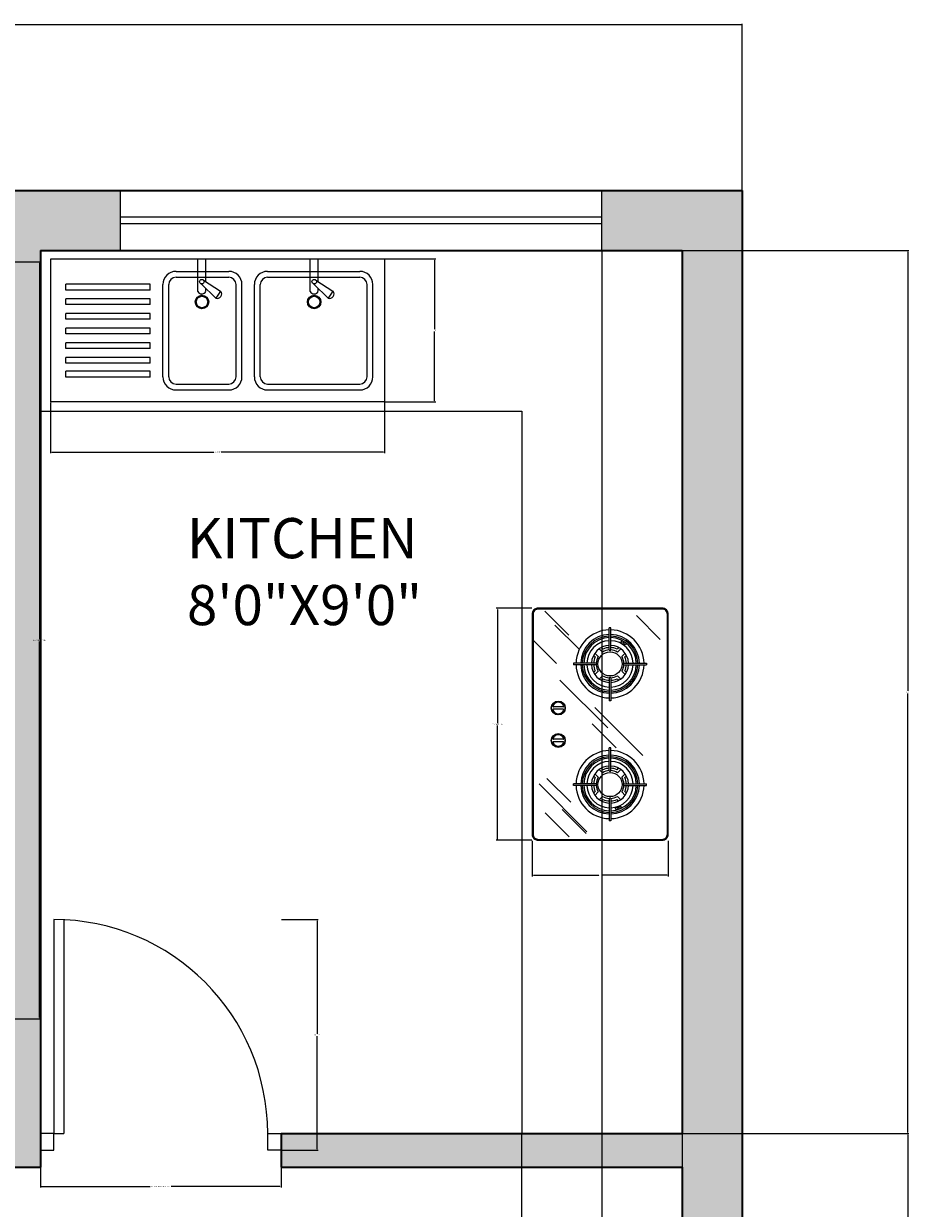
# Model space of a CAD drawing. Units: inches. Extents: x 126 to 477, y -70 to 465.
# Tile 5 of 5: x 344 to 477, y 288 to 465. Entities that reach past the tile are written whole.
import ezdxf

# ---------------------------------------------------------------- set-up
doc = ezdxf.new("R2010")
doc.units = ezdxf.units.IN
for name, color, linetype, lineweight in [('A-ANNO-DIMS', 2, 'Continuous', 18), ('A-AREA-IDEN', 7, 'Continuous', 20), ('A-DOOR', 4, 'Continuous', 20), ('A-EQPM', 9, 'Continuous', 18), ('A-FLOR-CASE', 8, 'Continuous', 25), ('A-FLOR-FIXT', 8, 'Continuous', 18), ('A-GLAZ', 4, 'Continuous', 18), ('A-WALL', 7, 'Continuous', 35), ('A-WALL-PATT', 252, 'Continuous', 13)]:
    doc.layers.add(name, color=color, linetype=linetype, lineweight=lineweight)
doc.styles.get("Standard").update_dxf_attribs({"font": 'arial.ttf'})
doc.dimstyles.get("Standard").update_dxf_attribs({"dimtxt": 0.18, "dimasz": 0.18, "dimexe": 0.18, "dimexo": 0.0625, "dimgap": 0.09, "dimtad": 0, "dimtih": 1, "dimtoh": 1, "dimdec": 4, "dimzin": 0, "dimdsep": 46, "dimtxsty": 'Standard', "dimcen": 0.09, "dimadec": 0, "dimazin": 0, "dimtfac": 1, "dimtdec": 4, "dimtofl": 0, "dimtmove": 0, "dimatfit": 3, "dimfxl": 1, "dimtolj": 1, "dimtzin": 0, "dimarcsym": 0})

# ---------------------------------------------------------------- blocks, each defined once
blk = doc.blocks.new('A$C6CB038CA')
for p, q in [((0, 0), (0, 488.5)), ((0, 488.5), (1140.7, 488.5)), ((502.8, 377.5), (502.8, 488.5)), ((529.8, 412.8), (529.8, 488.5)), ((886.8, 377.5), (886.8, 488.5)), ((913.8, 412.8), (913.8, 488.5)), ((1140.7, 488.5), (1140.7, 0)), ((428.4, 445.8), (608.4, 445.8)), ((740.8, 445.8), (1055.8, 445.8)), ((428.4, 425.8), (608.4, 425.8)), ((521.9, 415.4), (580.3, 378.4)), ((740.8, 425.8), (1055.8, 425.8)), ((906, 415.4), (964.3, 378.4)), ((52.2, 382.1), (52.2, 402.1)), ((339.4, 402.1), (52.2, 402.1)), ((339.4, 382.1), (52.2, 382.1)), ((339.4, 382.1), (339.4, 402.1)), ((383.4, 85.8), (383.4, 400.8)), ((403.4, 85.8), (403.4, 400.8)), ((563.7, 353.9), (514.9, 402.4)), ((529.8, 377.6), (529.8, 387.6)), ((580.3, 378.4), (563.7, 353.9)), ((633.4, 85.8), (633.4, 400.8)), ((653.4, 85.8), (653.4, 400.8)), ((695.8, 85.8), (695.8, 400.8)), ((715.8, 85.8), (715.8, 400.8)), ((947.8, 353.9), (899, 402.4)), ((913.8, 377.6), (913.8, 387.6)), ((964.3, 378.4), (947.8, 353.9)), ((1080.8, 85.8), (1080.8, 400.8)), ((1100.8, 85.8), (1100.8, 400.8)), ((52.2, 332.1), (52.2, 352.1)), ((339.4, 352.1), (52.2, 352.1)), ((339.4, 332.1), (52.2, 332.1)), ((339.4, 332.1), (339.4, 352.1)), ((52.2, 282.1), (52.2, 302.1)), ((339.4, 302.1), (52.2, 302.1)), ((339.4, 282.1), (339.4, 302.1)), ((339.4, 282.1), (52.2, 282.1)), ((52.2, 232.1), (52.2, 252.1)), ((339.4, 252.1), (52.2, 252.1)), ((339.4, 232.1), (339.4, 252.1)), ((339.4, 232.1), (52.2, 232.1)), ((52.2, 182.1), (52.2, 202.1)), ((339.4, 202.1), (52.2, 202.1)), ((339.4, 182.1), (52.2, 182.1)), ((339.4, 182.1), (339.4, 202.1)), ((52.2, 132.1), (52.2, 152.1)), ((339.4, 152.1), (52.2, 152.1)), ((339.4, 132.1), (52.2, 132.1)), ((339.4, 132.1), (339.4, 152.1)), ((52.2, 84.8), (52.2, 104.8)), ((339.4, 104.8), (52.2, 104.8)), ((339.4, 84.8), (52.2, 84.8)), ((339.4, 84.8), (339.4, 104.8)), ((428.4, 60.8), (608.4, 60.8)), ((428.4, 40.8), (608.4, 40.8)), ((740.8, 60.8), (1055.8, 60.8)), ((740.8, 40.8), (1055.8, 40.8)), ((1140.7, 0), (0, 0))]:
    blk.add_line(p, q)
for centre, radius in [((516.4, 410.5), 7.79), ((900.5, 410.5), 7.79), ((516.9, 341.2), 23.1), ((900.1, 341.2), 23.1), ((516.9, 341.3), 19.5), ((900.2, 341.3), 19.5)]:
    blk.add_circle(centre, radius)
for centre, radius, start, end in [((428.4, 400.8), 45, 90, 180), ((608.4, 400.8), 45, 0, 90), ((740.8, 400.8), 45, 90, 180), ((1055.8, 400.8), 45, 0, 90), ((428.4, 400.8), 25, 90, 180), ((608.4, 400.8), 25, 0, 90), ((740.8, 400.8), 25, 90, 180), ((1055.8, 400.8), 25, 0, 90), ((516.1, 383.8), 14.9, 205.1043, 335.2171), ((568.7, 368.6), 15.5, 251.2024, 39.3215), ((900.1, 383.8), 14.9, 205.1043, 335.2171), ((952.8, 368.6), 15.5, 251.2024, 39.3215), ((428.4, 85.8), 45, 180, 270), ((428.4, 85.8), 25, 180, 270), ((608.4, 85.8), 25, 270, 0), ((608.4, 85.8), 45, 270, 0), ((740.8, 85.8), 45, 180, 270), ((740.8, 85.8), 25, 180, 270), ((1055.8, 85.8), 25, 270, 0), ((1055.8, 85.8), 45, 270, 0)]:
    blk.add_arc(centre, radius, start, end)
blk = doc.blocks.new('A$C48FA29D1')
for p, q in [((23.9, 336.8), (101.3, 414.2)), ((177.6, 369.5), (182.6, 369.5)), ((320.9, 202.7), (475.7, 357.5)), ((572.4, 369.5), (567.4, 369.5)), ((374.2, 193.8), (451.6, 271.2)), ((63.2, 254.2), (63.2, 249.2)), ((232.1, 89.3), (386.9, 244.1)), ((299, 254.2), (299, 249.2)), ((451, 254.2), (451, 249.2)), ((686.8, 254.2), (686.8, 249.2)), ((567.6, 22.2), (722.4, 177)), ((650.5, 97.2), (727.9, 174.6)), ((10.1, 41), (87.5, 118.4)), ((54.5, 73.5), (131.9, 150.9)), ((177.6, 133.3), (182.6, 133.3)), ((549.9, 47.9), (627.2, 125.3)), ((572.4, 133.3), (567.4, 133.3)), ((661.4, 42), (738.7, 119.3)), ((100.9, 1.5), (178.3, 78.9))]:
    blk.add_line(p, q)
at = {"ltscale": 0.18}
for p, q in [((177.6, 296.7), (177.6, 369.5)), ((182.6, 296.7), (182.6, 369.5)), ((567.4, 296.7), (567.4, 369.5)), ((572.4, 296.7), (572.4, 369.5)), ((126.9, 279.5), (132.1, 274.3)), ((131.2, 286.5), (142, 275.7)), ((145.3, 300.6), (156.1, 289.8)), ((152.3, 304.9), (157.6, 299.7)), ((202.6, 299.7), (207.8, 304.9)), ((204, 289.8), (214.8, 300.6)), ((218.2, 275.7), (229, 286.5)), ((228.1, 274.3), (233.3, 279.5)), ((521.9, 274.3), (516.7, 279.5)), ((531.8, 275.7), (521, 286.5)), ((546, 289.8), (535.2, 300.6)), ((547.4, 299.7), (542.2, 304.9)), ((597.7, 304.9), (592.4, 299.7)), ((604.7, 300.6), (593.9, 289.8)), ((618.8, 286.5), (608, 275.7)), ((623.1, 279.5), (617.9, 274.3)), ((135.1, 254.2), (63.2, 254.2)), ((135.1, 249.2), (63.2, 249.2)), ((225, 254.2), (299, 254.2)), ((225, 249.2), (299, 249.2)), ((525, 254.2), (451, 254.2)), ((525, 249.2), (451, 249.2)), ((614.9, 254.2), (686.8, 254.2)), ((614.9, 249.2), (686.8, 249.2)), ((126.9, 224), (132.1, 229.2)), ((131.2, 217), (142, 227.8)), ((145.3, 202.8), (156.1, 213.6)), ((152.3, 198.5), (157.6, 203.8)), ((177.6, 206.8), (177.6, 133.3)), ((182.6, 206.8), (182.6, 133.3)), ((202.6, 203.8), (207.8, 198.5)), ((204, 213.6), (214.8, 202.8)), ((218.2, 227.8), (229, 217)), ((228.1, 229.2), (233.3, 224)), ((521.9, 229.2), (516.7, 224)), ((531.8, 227.8), (521, 217)), ((546, 213.6), (535.2, 202.8)), ((547.4, 203.8), (542.2, 198.5)), ((567.4, 206.8), (567.4, 133.3)), ((572.4, 206.8), (572.4, 133.3)), ((597.7, 198.5), (592.4, 203.8)), ((604.7, 202.8), (593.9, 213.6)), ((618.8, 217), (608, 227.8)), ((623.1, 224), (617.9, 229.2)), ((318.6, 99.8), (318.6, 69)), ((326.6, 99.8), (326.6, 69)), ((423.4, 99.8), (423.4, 69)), ((431.4, 99.8), (431.4, 69))]:
    blk.add_line(p, q, dxfattribs=at)
for points in [[(20, 0), (730, 0, 0.414214), (750, 20), (750, 420, 0.414214), (730, 440), (20, 440, 0.414214), (0, 420), (0, 20, 0.414214)], [(20, 3), (730, 3, 0.414214), (747, 20), (747, 420, 0.414214), (730, 437), (20, 437, 0.414214), (3, 420), (3, 20, 0.414214)]]:
    blk.add_lwpolyline(points, format="xyb", close=True)
for centre in [(109.4, 291.3), (115.3, 300.3), (642.8, 283.6), (646.9, 273)]:
    blk.add_circle(centre, 3.58)
for centre, radius in [((180.1, 251.7), 39), ((569.9, 251.7), 39), ((322.6, 84.4), 22.5), ((322.6, 84.4), 21.5), ((427.4, 84.4), 22.5), ((427.4, 84.4), 21.5)]:
    blk.add_circle(centre, radius, dxfattribs=at)
for centre, radius, start, end in [((180.1, 251.7), 110, 91.3023, 178.6977), ((180.1, 251.7), 95, 91.5918, 178.4082), ((180.1, 251.7), 110, 1.3023, 88.6977), ((180.1, 251.7), 95, 1.5918, 88.4082), ((569.9, 251.7), 110, 91.3023, 178.6977), ((569.9, 251.7), 95, 91.5918, 178.4082), ((569.9, 251.7), 110, 1.3023, 88.6977), ((569.9, 251.7), 95, 1.5918, 88.4082), ((180.1, 251.7), 90, 91.5918, 178.4082), ((180.1, 251.7), 85, 91.6854, 178.3146), ((180.1, 251.7), 75, 91.9102, 178.0898), ((180.1, 251.7), 60, 92.388, 177.612), ((180.1, 251.7), 90, 1.5918, 88.4082), ((180.1, 251.7), 85, 1.6854, 88.3146), ((180.1, 251.7), 75, 1.9102, 88.0898), ((180.1, 251.7), 60, 2.388, 87.612), ((569.9, 251.7), 90, 91.5918, 178.4082), ((569.9, 251.7), 85, 91.6854, 178.3146), ((569.9, 251.7), 75, 91.9102, 178.0898), ((569.9, 251.7), 60, 92.388, 177.612), ((569.9, 251.7), 90, 1.5918, 88.4082), ((569.9, 251.7), 85, 1.6854, 88.3146), ((569.9, 251.7), 75, 1.9102, 88.0898), ((569.9, 251.7), 60, 2.388, 87.612), ((180.1, 251.7), 53, 154.8539, 177.2964), ((180.1, 251.7), 45, 147.8396, 176.8153), ((180.1, 251.7), 45, 93.1847, 122.1604), ((180.1, 251.7), 53, 92.7036, 115.1461), ((180.1, 297), 2.52, 186.7354, 353.2646), ((180.1, 251.7), 53, 64.8539, 87.2964), ((180.1, 251.7), 45, 57.8396, 86.8153), ((180.1, 251.7), 45, 3.1847, 32.1604), ((180.1, 251.7), 53, 2.7036, 25.1461), ((569.9, 251.7), 53, 154.8539, 177.2964), ((569.9, 251.7), 45, 147.8396, 176.8153), ((569.9, 251.7), 45, 93.1847, 122.1604), ((569.9, 251.7), 53, 92.7036, 115.1461), ((569.9, 296.8), 2.51, 183.9579, 356.0421), ((569.9, 251.7), 53, 64.8539, 87.2964), ((569.9, 251.7), 45, 57.8396, 86.8153), ((569.9, 251.7), 45, 3.1847, 32.1604), ((569.9, 251.7), 53, 2.7036, 25.1461), ((180.1, 251.7), 110, 181.3023, 268.6977), ((180.1, 251.7), 95, 181.5918, 268.4082), ((180.1, 251.7), 90, 181.5918, 268.4082), ((180.1, 251.7), 85, 181.6854, 268.3146), ((180.1, 251.7), 75, 181.9102, 268.0898), ((180.1, 251.7), 60, 182.388, 267.612), ((180.1, 251.7), 53, 182.7036, 205.1461), ((134.3, 251.7), 2.64, 288.751, 71.249), ((180.1, 251.7), 45, 183.1847, 212.1604), ((180.1, 251.7), 90, 271.5918, 358.4082), ((180.1, 251.7), 85, 271.6854, 358.3146), ((180.1, 251.7), 110, 271.3023, 358.6977), ((180.1, 251.7), 75, 271.9102, 358.0898), ((180.1, 251.7), 60, 272.388, 357.612), ((180.1, 251.7), 95, 271.5918, 358.4082), ((180.1, 251.7), 45, 327.8396, 356.8153), ((225.9, 251.7), 2.67, 110.5507, 249.4493), ((180.1, 251.7), 53, 334.8539, 357.2964), ((569.9, 251.7), 110, 181.3023, 268.6977), ((569.9, 251.7), 95, 181.5918, 268.4082), ((569.9, 251.7), 90, 181.5918, 268.4082), ((569.9, 251.7), 85, 181.6854, 268.3146), ((569.9, 251.7), 75, 181.9102, 268.0898), ((569.9, 251.7), 60, 182.388, 267.612), ((569.9, 251.7), 53, 182.7036, 205.1461), ((524.2, 251.7), 2.63, 288.412, 71.588), ((569.9, 251.7), 45, 183.1847, 212.1604), ((569.9, 251.7), 75, 271.9102, 358.0898), ((569.9, 251.7), 85, 271.6854, 358.3146), ((569.9, 251.7), 110, 271.3023, 358.6977), ((569.9, 251.7), 90, 271.5918, 358.4082), ((569.9, 251.7), 60, 272.388, 357.612), ((569.9, 251.7), 95, 271.5918, 358.4082), ((569.9, 251.7), 45, 327.8396, 356.8153), ((615.5, 251.7), 2.58, 104.2945, 255.7055), ((569.9, 251.7), 53, 334.8539, 357.2964), ((180.1, 251.7), 45, 237.8396, 266.8153), ((180.1, 251.7), 53, 244.8539, 267.2964), ((180.1, 205.8), 2.69, 21.7885, 158.2115), ((180.1, 251.7), 45, 273.1847, 302.1604), ((180.1, 251.7), 53, 272.7036, 295.1461), ((569.9, 251.7), 45, 237.8396, 266.8153), ((569.9, 251.7), 53, 244.8539, 267.2964), ((569.9, 206), 2.63, 17.9418, 162.0582), ((569.9, 251.7), 45, 273.1847, 302.1604), ((569.9, 251.7), 53, 272.7036, 295.1461), ((322.6, 84.4), 18.5, 111.3237, 248.6763), ((316.6, 99.8), 2, 0, 111.3237), ((328.6, 99.8), 2, 68.6763, 180), ((322.6, 84.4), 18.5, 291.3237, 68.6763), ((427.4, 84.4), 18.5, 111.3237, 248.6763), ((421.4, 99.8), 2, 0, 111.3237), ((433.4, 99.8), 2, 68.6763, 180), ((427.4, 84.4), 18.5, 291.3237, 68.6763), ((316.6, 69), 2, 248.6763, 0), ((328.6, 69), 2, 180, 291.3237), ((421.4, 69), 2, 248.6763, 0), ((433.4, 69), 2, 180, 291.3237)]:
    blk.add_arc(centre, radius, start, end, dxfattribs=at)
blk = doc.blocks.new('DOOR-SINGLE-36IN')
for p, q in [((2, 34.5), (2, 2.5)), ((3.5, 34.46), (3.5, 2.5)), ((2, 2.5), (0, 2.5)), ((2, 0), (2, 2.5)), ((2, 2.5), (3.5, 2.5)), ((34, 0), (34, 2.5)), ((34, 2.5), (36, 2.5)), ((0, 0), (2, 0)), ((36, 0), (34, 0))]:
    blk.add_line(p, q)
blk.add_arc((2, 2.5), 32, 0, 90)
blk = doc.blocks.new('WIN-72IN')
for p, q in [((0, 0), (0, 9)), ((72, 0), (72, 9)), ((72, 5), (0, 5)), ((72, 4), (0, 4))]:
    blk.add_line(p, q)
blk = doc.blocks.new('*D13')
at = {"layer": 'A-ANNO-DIMS', "color": 0, "lineweight": -2, "transparency": 16777216}
for p, q in [((346.53, 296.32), (346.53, 290.8)), ((382.53, 296.32), (382.53, 290.8)), ((346.71, 290.98), (362.96, 290.98)), ((382.35, 290.98), (366.1, 290.98))]:
    blk.add_line(p, q, dxfattribs=at)
at = {"layer": 'A-ANNO-DIMS', "color": 0, "transparency": 16777216}
for points in [[(346.71, 291.01), (346.71, 290.95), (346.53, 290.98)], [(382.35, 291.01), (382.35, 290.95), (382.53, 290.98)]]:
    blk.add_solid(points, dxfattribs=at)
at = {"layer": 'Defpoints', "color": 0, "transparency": 16777216}
for p in [(346.53, 296.38), (382.53, 296.38), (382.53, 290.98)]:
    blk.add_point(p, dxfattribs=at)
at = {"layer": 'A-ANNO-DIMS', "color": 0, "transparency": 16777216, "insert": (364.53, 290.98), "char_height": 0.18, "attachment_point": 5}
blk.add_mtext('\\A1;INTERIOR DOOR 36 TYP.', dxfattribs=at)
blk = doc.blocks.new('*D14')
at = {"layer": 'A-ANNO-DIMS', "color": 0, "lineweight": -2, "transparency": 16777216}
for p, q in [((382.6, 330.88), (388.11, 330.88)), ((387.93, 330.7), (387.93, 313.81)), ((387.93, 296.56), (387.93, 313.45)), ((382.6, 296.38), (388.11, 296.38))]:
    blk.add_line(p, q, dxfattribs=at)
at = {"layer": 'A-ANNO-DIMS', "color": 0, "transparency": 16777216}
for points in [[(387.9, 330.7), (387.96, 330.7), (387.93, 330.88)], [(387.9, 296.56), (387.96, 296.56), (387.93, 296.38)]]:
    blk.add_solid(points, dxfattribs=at)
at = {"layer": 'Defpoints', "color": 0, "transparency": 16777216}
for p in [(382.53, 330.88), (387.93, 330.88), (382.53, 296.38)]:
    blk.add_point(p, dxfattribs=at)
at = {"layer": 'A-ANNO-DIMS', "color": 0, "transparency": 16777216, "insert": (387.93, 313.63), "char_height": 0.18, "attachment_point": 5}
blk.add_mtext('\\A1;35 TYP.', dxfattribs=at)
blk = doc.blocks.new('*D19')
at = {"layer": 'A-ANNO-DIMS', "color": 0, "lineweight": -2, "transparency": 16777216}
for p, q in [((329.49, 429.2), (346.57, 429.2)), ((346.39, 429.02), (346.39, 372.81)), ((346.39, 316.23), (346.39, 372.44)), ((329.49, 316.05), (346.57, 316.05))]:
    blk.add_line(p, q, dxfattribs=at)
at = {"layer": 'A-ANNO-DIMS', "color": 0, "transparency": 16777216}
for points in [[(346.36, 429.02), (346.42, 429.02), (346.39, 429.2)], [(346.36, 316.23), (346.42, 316.23), (346.39, 316.05)]]:
    blk.add_solid(points, dxfattribs=at)
at = {"layer": 'Defpoints', "color": 0, "transparency": 16777216}
for p in [(329.42, 429.2), (346.39, 429.2), (329.42, 316.05)]:
    blk.add_point(p, dxfattribs=at)
at = {"layer": 'A-ANNO-DIMS', "color": 0, "transparency": 16777216, "insert": (346.39, 372.63), "char_height": 0.18, "attachment_point": 5}
blk.add_mtext('\\A1;BED GROUP 113', dxfattribs=at)
blk = doc.blocks.new('*D21')
at = {"layer": 'A-ANNO-DIMS', "color": 0, "lineweight": -2, "transparency": 16777216}
for p, q in [((348.07, 408.2), (348.07, 400.59)), ((398.02, 408.2), (398.02, 400.59)), ((348.25, 400.77), (372.5, 400.77)), ((397.84, 400.77), (373.59, 400.77))]:
    blk.add_line(p, q, dxfattribs=at)
at = {"layer": 'A-ANNO-DIMS', "color": 0, "transparency": 16777216}
for points in [[(348.25, 400.8), (348.25, 400.74), (348.07, 400.77)], [(397.84, 400.8), (397.84, 400.74), (398.02, 400.77)]]:
    blk.add_solid(points, dxfattribs=at)
at = {"layer": 'Defpoints', "color": 0, "transparency": 16777216}
for p in [(348.07, 408.26), (398.02, 408.26), (398.02, 400.77)]:
    blk.add_point(p, dxfattribs=at)
at = {"layer": 'A-ANNO-DIMS', "color": 0, "transparency": 16777216, "insert": (373.05, 400.77), "char_height": 0.18, "attachment_point": 5}
blk.add_mtext('\\A1;SINK 50', dxfattribs=at)
blk = doc.blocks.new('*D22')
at = {"layer": 'A-ANNO-DIMS', "color": 0, "lineweight": -2, "transparency": 16777216}
for p, q in [((398.08, 429.66), (405.69, 429.66)), ((405.51, 429.48), (405.51, 419.14)), ((405.51, 408.44), (405.51, 418.78)), ((398.08, 408.26), (405.69, 408.26))]:
    blk.add_line(p, q, dxfattribs=at)
at = {"layer": 'A-ANNO-DIMS', "color": 0, "transparency": 16777216}
for points in [[(405.48, 429.48), (405.54, 429.48), (405.51, 429.66)], [(405.48, 408.44), (405.54, 408.44), (405.51, 408.26)]]:
    blk.add_solid(points, dxfattribs=at)
at = {"layer": 'Defpoints', "color": 0, "transparency": 16777216}
for p in [(398.02, 429.66), (405.51, 429.66), (398.02, 408.26)]:
    blk.add_point(p, dxfattribs=at)
at = {"layer": 'A-ANNO-DIMS', "color": 0, "transparency": 16777216, "insert": (405.51, 418.96), "char_height": 0.18, "attachment_point": 5}
blk.add_mtext('\\A1;21', dxfattribs=at)
blk = doc.blocks.new('*D23')
at = {"layer": 'A-ANNO-DIMS', "color": 0, "lineweight": -2, "transparency": 16777216}
for p, q in [((420.04, 377.43), (414.72, 377.43)), ((414.9, 377.25), (414.9, 360.26)), ((414.9, 342.91), (414.9, 359.9)), ((420.04, 342.73), (414.72, 342.73))]:
    blk.add_line(p, q, dxfattribs=at)
at = {"layer": 'A-ANNO-DIMS', "color": 0, "transparency": 16777216}
for points in [[(414.87, 377.25), (414.93, 377.25), (414.9, 377.43)], [(414.87, 342.91), (414.93, 342.91), (414.9, 342.73)]]:
    blk.add_solid(points, dxfattribs=at)
at = {"layer": 'Defpoints', "color": 0, "transparency": 16777216}
for p in [(420.1, 377.43), (414.9, 342.73), (420.1, 342.73)]:
    blk.add_point(p, dxfattribs=at)
at = {"layer": 'A-ANNO-DIMS', "color": 0, "transparency": 16777216, "insert": (414.9, 360.08), "char_height": 0.18, "attachment_point": 5}
blk.add_mtext('\\A1;COOKTOP 35', dxfattribs=at)
blk = doc.blocks.new('*D24')
at = {"layer": 'A-ANNO-DIMS', "color": 0, "lineweight": -2, "transparency": 16777216}
for p, q in [((420.1, 342.66), (420.1, 337.34)), ((440.47, 342.66), (440.47, 337.34)), ((420.28, 337.52), (430.06, 337.52)), ((440.29, 337.52), (430.5, 337.52))]:
    blk.add_line(p, q, dxfattribs=at)
at = {"layer": 'A-ANNO-DIMS', "color": 0, "transparency": 16777216}
for points in [[(420.28, 337.55), (420.28, 337.49), (420.1, 337.52)], [(440.29, 337.55), (440.29, 337.49), (440.47, 337.52)]]:
    blk.add_solid(points, dxfattribs=at)
at = {"layer": 'Defpoints', "color": 0, "transparency": 16777216}
for p in [(420.1, 342.73), (440.47, 342.73), (440.47, 337.52)]:
    blk.add_point(p, dxfattribs=at)
at = {"layer": 'A-ANNO-DIMS', "color": 0, "transparency": 16777216, "insert": (430.28, 337.52), "char_height": 0.18, "attachment_point": 5}
blk.add_mtext('\\A1;20', dxfattribs=at)
blk = doc.blocks.new('*D29')
at = {"layer": 'A-ANNO-DIMS', "color": 0, "lineweight": -2, "transparency": 16777216}
for p, q in [((200.53, 439.94), (200.53, 464.81)), ((200.71, 464.63), (325.76, 464.63)), ((451.35, 464.63), (326.31, 464.63)), ((451.53, 439.94), (451.53, 464.81))]:
    blk.add_line(p, q, dxfattribs=at)
at = {"layer": 'A-ANNO-DIMS', "color": 0, "transparency": 16777216}
for points in [[(200.71, 464.66), (200.71, 464.6), (200.53, 464.63)], [(451.35, 464.66), (451.35, 464.6), (451.53, 464.63)]]:
    blk.add_solid(points, dxfattribs=at)
at = {"layer": 'Defpoints', "color": 0, "transparency": 16777216}
for p in [(451.53, 464.63), (200.53, 439.88), (451.53, 439.88)]:
    blk.add_point(p, dxfattribs=at)
at = {"layer": 'A-ANNO-DIMS', "color": 0, "transparency": 16777216, "insert": (326.03, 464.63), "char_height": 0.18, "attachment_point": 5}
blk.add_mtext('\\A1;251', dxfattribs=at)
blk = doc.blocks.new('*D32')
at = {"layer": 'A-ANNO-DIMS', "color": 0, "lineweight": -2, "transparency": 16777216}
for p, q in [((430.53, 430.82), (430.53, -70.05)), ((442.53, 430.82), (442.53, -70.05)), ((430.71, -69.87), (436.32, -69.87)), ((442.35, -69.87), (436.74, -69.87))]:
    blk.add_line(p, q, dxfattribs=at)
at = {"layer": 'A-ANNO-DIMS', "color": 0, "transparency": 16777216}
for points in [[(430.71, -69.84), (430.71, -69.9), (430.53, -69.87)], [(442.35, -69.84), (442.35, -69.9), (442.53, -69.87)]]:
    blk.add_solid(points, dxfattribs=at)
at = {"layer": 'Defpoints', "color": 0, "transparency": 16777216}
for p in [(430.53, 430.88), (442.53, 430.88), (442.53, -69.87)]:
    blk.add_point(p, dxfattribs=at)
at = {"layer": 'A-ANNO-DIMS', "color": 0, "transparency": 16777216, "insert": (436.53, -69.87), "char_height": 0.18, "attachment_point": 5}
blk.add_mtext('\\A1;12', dxfattribs=at)
blk = doc.blocks.new('*D37')
at = {"layer": 'A-ANNO-DIMS', "color": 0, "lineweight": -2, "transparency": 16777216}
for p, q in [((442.6, 298.88), (476.46, 298.88)), ((476.28, 298.7), (476.28, 265.81)), ((476.28, 232.56), (476.28, 265.45)), ((451.6, 232.38), (476.46, 232.38))]:
    blk.add_line(p, q, dxfattribs=at)
at = {"layer": 'A-ANNO-DIMS', "color": 0, "transparency": 16777216}
for points in [[(476.25, 298.7), (476.31, 298.7), (476.28, 298.88)], [(476.25, 232.56), (476.31, 232.56), (476.28, 232.38)]]:
    blk.add_solid(points, dxfattribs=at)
at = {"layer": 'Defpoints', "color": 0, "transparency": 16777216}
for p in [(442.53, 298.88), (476.28, 298.88), (451.53, 232.38)]:
    blk.add_point(p, dxfattribs=at)
at = {"layer": 'A-ANNO-DIMS', "color": 0, "transparency": 16777216, "insert": (476.28, 265.63), "char_height": 0.18, "attachment_point": 5}
blk.add_mtext('\\A1;66.5', dxfattribs=at)
blk = doc.blocks.new('*D38')
at = {"layer": 'A-ANNO-DIMS', "color": 0, "lineweight": -2, "transparency": 16777216}
for p, q in [((442.6, 430.88), (476.46, 430.88)), ((476.28, 430.7), (476.28, 365.06)), ((476.28, 299.06), (476.28, 364.7)), ((442.6, 298.88), (476.46, 298.88))]:
    blk.add_line(p, q, dxfattribs=at)
at = {"layer": 'A-ANNO-DIMS', "color": 0, "transparency": 16777216}
for points in [[(476.25, 430.7), (476.31, 430.7), (476.28, 430.88)], [(476.25, 299.06), (476.31, 299.06), (476.28, 298.88)]]:
    blk.add_solid(points, dxfattribs=at)
at = {"layer": 'Defpoints', "color": 0, "transparency": 16777216}
for p in [(442.53, 430.88), (476.28, 430.88), (442.53, 298.88)]:
    blk.add_point(p, dxfattribs=at)
at = {"layer": 'A-ANNO-DIMS', "color": 0, "transparency": 16777216, "insert": (476.28, 364.88), "char_height": 0.18, "attachment_point": 5}
blk.add_mtext('\\A1;132', dxfattribs=at)
blk = doc.blocks.new('*D48')
at = {"layer": 'A-ANNO-DIMS', "color": 0, "lineweight": -2, "transparency": 16777216}
for p, q in [((418.53, 298.82), (418.53, -70.05)), ((442.53, 298.82), (442.53, -70.05)), ((418.71, -69.87), (430.31, -69.87)), ((442.35, -69.87), (430.75, -69.87))]:
    blk.add_line(p, q, dxfattribs=at)
at = {"layer": 'A-ANNO-DIMS', "color": 0, "transparency": 16777216}
for points in [[(418.71, -69.84), (418.71, -69.9), (418.53, -69.87)], [(442.35, -69.84), (442.35, -69.9), (442.53, -69.87)]]:
    blk.add_solid(points, dxfattribs=at)
at = {"layer": 'Defpoints', "color": 0, "transparency": 16777216}
for p in [(418.53, 298.88), (442.53, 298.88), (442.53, -69.87)]:
    blk.add_point(p, dxfattribs=at)
at = {"layer": 'A-ANNO-DIMS', "color": 0, "transparency": 16777216, "insert": (430.53, -69.87), "char_height": 0.18, "attachment_point": 5}
blk.add_mtext('\\A1;24', dxfattribs=at)

msp = doc.modelspace()

# ---------------------------------------------------------------- hatches: boundary and pattern name
at = {"layer": 'A-WALL-PATT'}
h = msp.add_hatch(color=256, dxfattribs=at)
h.dxf.hatch_style = 1
h.paths.add_polyline_path([(346.5333, 430.8806), (358.5333, 430.8806), (358.5333, 439.8806), (311.5333, 439.8806), (311.5333, 430.8806), (341.5333, 430.8806), (341.5333, 293.8806), (346.5333, 293.8806)])
h = msp.add_hatch(color=256, dxfattribs=at)
h.dxf.hatch_style = 1
h.paths.add_polyline_path([(451.5333, 439.8806), (430.5333, 439.8806), (430.5333, 430.8806), (442.5333, 430.8806), (442.5333, 298.8806), (382.5333, 298.8806), (382.5333, 293.8806), (442.5333, 293.8806), (442.5333, 232.3806), (451.5333, 232.3806)])

# ---------------------------------------------------------------- linework, layer by layer
at = {"layer": 'A-FLOR-CASE'}
for p, q in [((346.5333, 406.8806), (418.5333, 406.8806)), ((418.5333, 406.8806), (418.5333, 298.8806))]:
    msp.add_line(p, q, dxfattribs=at)
at = {"layer": 'A-WALL'}
for p, q in [((200.5333, 439.8806), (451.5333, 439.8806)), ((451.5333, 439.8806), (451.5333, -45.1194)), ((346.5333, 430.8806), (346.5333, 293.8806)), ((346.5333, 430.8806), (442.5333, 430.8806)), ((442.5333, 430.8806), (442.5333, 298.8806)), ((382.5333, 298.8806), (442.5333, 298.8806)), ((382.5333, 298.8806), (382.5333, 293.8806)), ((341.5333, 293.8806), (346.5333, 293.8806)), ((382.5333, 293.8806), (442.5333, 293.8806)), ((442.5333, 293.8806), (442.5333, 98.8806))]:
    msp.add_line(p, q, dxfattribs=at)

# ---------------------------------------------------------------- block references
at = {"layer": 'A-DOOR'}
msp.add_blockref('DOOR-SINGLE-36IN', (346.5333, 296.3806), dxfattribs=at)
at = {"layer": 'A-EQPM', "xscale": 0.0462772810747846, "yscale": 0.0462772810747846, "zscale": 0.0462772810747846, "rotation": 270}
msp.add_blockref('A$C48FA29D1', (420.1033, 377.4343), dxfattribs=at)
at = {"layer": 'A-FLOR-FIXT', "xscale": 0.0437891121363003, "yscale": 0.0437891121363003, "zscale": 0.0437891121363003}
msp.add_blockref('A$C6CB038CA', (348.0721, 408.2643), dxfattribs=at)
at = {"layer": 'A-GLAZ'}
msp.add_blockref('WIN-72IN', (358.5333, 430.8806), dxfattribs=at)

# ---------------------------------------------------------------- texts
at = {"layer": 'A-AREA-IDEN', "insert": (368.4592, 390.8972), "char_height": 6, "attachment_point": 1}
msp.add_mtext_dynamic_manual_height_columns('KITCHEN\\P8\'0"X9\'0"', width=74.074101, gutter_width=12.5, heights=[0], dxfattribs=at)

# ---------------------------------------------------------------- dimensions: what is measured, and where the dimension line sits
at = {"layer": 'A-ANNO-DIMS'}
for base, p1, p2, picture, middle in [((451.5333, 464.6306), (200.5333, 439.8806), (451.5333, 439.8806), '*D29', (326.0333, 464.6306)), ((442.5333, -69.8694), (430.5333, 430.8806), (442.5333, 430.8806), '*D32', (436.5333, -69.8694)), ((440.4653, 337.5202), (420.1033, 342.7264), (440.4653, 342.7264), '*D24', (430.2843, 337.5202)), ((442.5333, -69.8694), (418.5333, 298.8806), (442.5333, 298.8806), '*D48', (430.5333, -69.8694))]:
    dim = msp.add_linear_dim(base=base, p1=p1, p2=p2, dimstyle='Standard', override={"dimdec": 0, "dimlfac": 1, "dimrnd": 0, "dimzin": 0, "dimdsep": 46, "dimlunit": 2}, dxfattribs=at)
    dim.commit()
    dim.dimension.update_dxf_attribs({"geometry": picture, "text_midpoint": middle})
for base, p1, p2, override, picture, middle in [((476.2833, 430.8806), (442.5333, 298.8806), (442.5333, 430.8806), {"dimdec": 0, "dimlfac": 1, "dimrnd": 0, "dimzin": 0, "dimdsep": 46, "dimlunit": 2}, '*D38', (476.2833, 364.8806)), ((405.5138, 429.6567), (398.0214, 408.2643), (398.0214, 429.6567), {"dimdec": 0, "dimlfac": 1, "dimrnd": 0, "dimzin": 0, "dimdsep": 46, "dimlunit": 2}, '*D22', (405.5138, 418.9605)), ((476.2833, 298.8806), (451.5333, 232.3806), (442.5333, 298.8806), {"dimdec": 1, "dimlfac": 1, "dimrnd": 0, "dimzin": 0, "dimdsep": 46, "dimlunit": 2}, '*D37', (476.2833, 265.6306))]:
    dim = msp.add_linear_dim(base=base, p1=p1, p2=p2, angle=90, dimstyle='Standard', override=override, dxfattribs=at)
    dim.commit()
    dim.dimension.update_dxf_attribs({"geometry": picture, "text_midpoint": middle})
for base, p1, p2, angle, text, picture, middle in [((346.3943, 429.1976), (329.4226, 316.0525), (329.4226, 429.1976), 90, 'BED GROUP <>', '*D19', (346.3943, 372.6251)), ((414.8971, 342.7264), (420.1033, 377.4343), (420.1033, 342.7264), 270, 'COOKTOP <>', '*D23', (414.8971, 360.0803)), ((387.9333001297, 330.8806461871), (382.5333001297, 296.3806461871), (382.5333001297, 330.8806461871), 90, '<> TYP.', '*D14', (387.9333001297, 313.6306461871))]:
    dim = msp.add_linear_dim(base=base, p1=p1, p2=p2, angle=angle, text=text, dimstyle='Standard', override={"dimdec": 0, "dimlfac": 1, "dimrnd": 0, "dimzin": 0, "dimdsep": 46, "dimlunit": 2}, dxfattribs=at)
    dim.commit()
    dim.dimension.update_dxf_attribs({"geometry": picture, "text_midpoint": middle})
for base, p1, p2, text, picture, middle in [((398.0214, 400.7719), (348.0721, 408.2643), (398.0214, 408.2643), 'SINK <>', '*D21', (373.0468, 400.7719)), ((382.5333, 290.9806), (346.5333, 296.3806), (382.5333, 296.3806), 'INTERIOR DOOR <> TYP.', '*D13', (364.5333, 290.9806))]:
    dim = msp.add_linear_dim(base=base, p1=p1, p2=p2, text=text, dimstyle='Standard', override={"dimdec": 0, "dimlfac": 1, "dimrnd": 0, "dimzin": 0, "dimdsep": 46, "dimlunit": 2}, dxfattribs=at)
    dim.commit()
    dim.dimension.update_dxf_attribs({"geometry": picture, "text_midpoint": middle})

doc.saveas('drawing.dxf')
